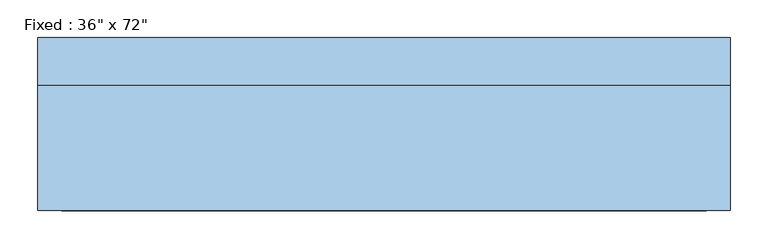
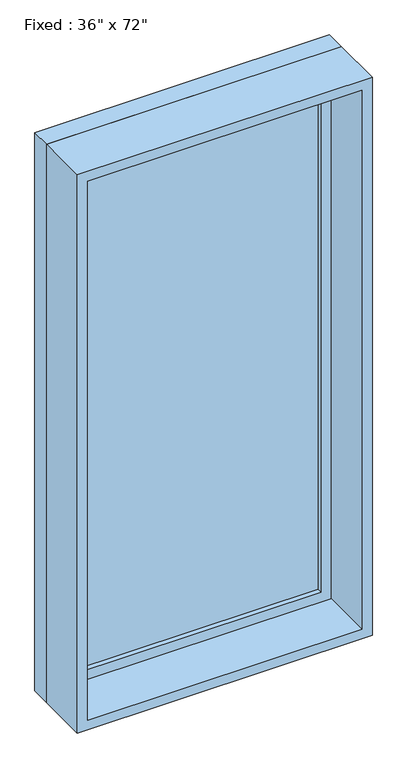
"""IFC4 building model written with IfcOpenShell, lengths in millimetres: window geometry."""

from ifc_helpers import new_model, si_unit, frame, origin, place, context, project, spatial, polyline, outline, extrude, source, transform, mapped, element, save


def window_c796fc87(model_context):
    return source(origin(), model_context, "Body", "SweptSolid", [
        extrude(outline(polyline([(355.6, 66.675), (-431.8, 66.675), (-431.8, 79.375), (355.6, 79.375), (355.6, 66.675)])), frame((0.0, 0.0, 368.3), z_axis=(0.0, 0.0, 1.0), x_axis=(1.0, 0.0, 0.0)), (0.0, 0.0, 1.0), 1701.8),
        extrude(outline(polyline([(2114.55, -476.25), (323.85, -476.25), (323.85, 400.05), (2114.55, 400.05), (2114.55, -476.25)]), holes=[polyline([(2070.1, -431.8), (2070.1, 355.6), (368.3, 355.6), (368.3, -431.8), (2070.1, -431.8)])]), frame((0.0, 50.8, 0.0), z_axis=(0.0, 1.0, 0.0), x_axis=(0.0, 0.0, 1.0)), (0.0, 0.0, 1.0), 44.45),
        extrude(outline(polyline([(2133.6, -495.3), (304.8, -495.3), (304.8, 419.1), (2133.6, 419.1), (2133.6, -495.3)]), holes=[polyline([(2101.85, -463.55), (2101.85, 387.35), (336.55, 387.35), (336.55, -463.55), (2101.85, -463.55)])]), frame((0.0, -114.3, 0.0), z_axis=(0.0, 1.0, 0.0), x_axis=(0.0, 0.0, 1.0)), (0.0, 0.0, 1.0), 165.1),
        extrude(outline(polyline([(2133.6, 419.1), (2133.6, -495.3), (304.8, -495.3), (304.8, 419.1), (2133.6, 419.1)]), holes=[polyline([(2114.55, 400.05), (323.85, 400.05), (323.85, -476.25), (2114.55, -476.25), (2114.55, 400.05)])]), frame((0.0, 50.8, 0.0), z_axis=(0.0, 1.0, 0.0), x_axis=(0.0, 0.0, 1.0)), (0.0, 0.0, 1.0), 63.5),
    ])


if __name__ == "__main__":
    model = new_model("IFC4")
    model_context = context("Model", 3, world=origin())
    ifc_project = project(units=[si_unit("LENGTHUNIT", "METRE", prefix="MILLI")], contexts=[model_context])
    site = spatial("IfcSite", under=ifc_project)
    building = spatial("IfcBuilding", under=site)
    placement = place(None, origin())
    window_shape = window_c796fc87(model_context)
    element("IfcWindow", 1, ObjectType="Fixed : 36\" x 72\"", at=placement, inside=building, context=model_context, shape_type="MappedRepresentation", body=[
        mapped(window_shape, transform((0.0, 0.0, 0.0), x_axis=(1.0, 0.0, 0.0), y_axis=(0.0, 1.0, 0.0), z_axis=(0.0, 0.0, 1.0))),
    ])
    save(model, "model.ifc")

# Revit data of these elements
# Type "Fixed : 36\" x 72\""
#   Type Mark = "9"
#   Assembly Code = "B2020100"
#   Height = 6' - 0"
#   Default Sill Height = 1' - 0"
#   Width = 3' - 0"
#   Window Inset = 0' - 0 3/4"
#   Glass Pane Material = Glass
#   Sash Material = Sash
#   Wall Closure = (empty or 0)
# Element 1 (IfcWindow, "Fixed : 36\" x 72\"")
#   Materials on its faces: "Sash", "Glass"
# Materials
#   "Glass": class "Glass", colour RGB 218 227 224, transparency 0.85, Description = "Soda Lime Glass", Cost = 0
#   "Sash": class "Wood", colour RGB 136 99 55, transparency 0
